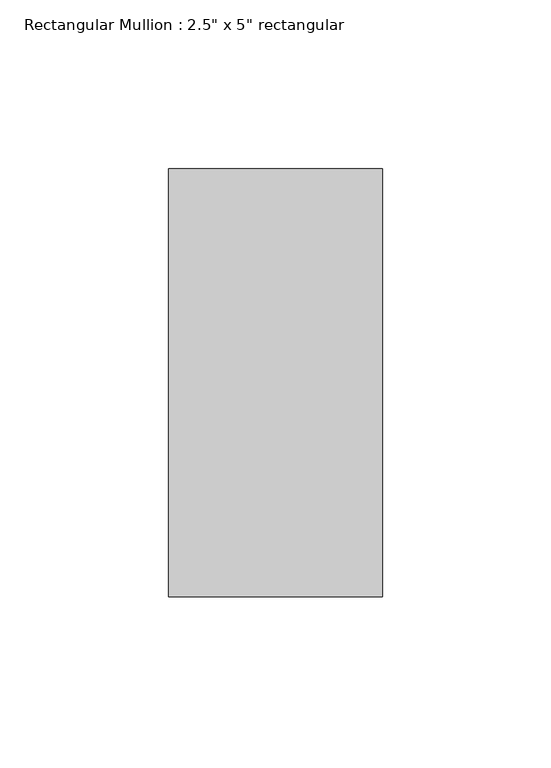
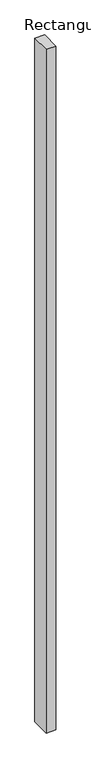
"""IFC4 building model written with IfcOpenShell, lengths in millimetres: member geometry."""

from ifc_helpers import new_model, si_unit, frame, origin, place, context, project, spatial, polyline, outline, extrude, source, transform, mapped, element, save


def member_bf9e663f(model_context):
    return source(origin(), model_context, "Body", "SweptSolid", [
        extrude(outline(polyline([(0.0, 63.5), (0.0, -63.5), (-63.5, -63.5), (-63.5, 63.5), (0.0, 63.5)])), frame((0.0, 0.0, -4736.2841492), z_axis=(0.0, 0.0, 1.0), x_axis=(1.0, 0.0, 0.0)), (0.0, 0.0, 1.0), 4736.2841492),
    ])


if __name__ == "__main__":
    model = new_model("IFC4")
    model_context = context("Model", 3, world=origin())
    ifc_project = project(units=[si_unit("LENGTHUNIT", "METRE", prefix="MILLI")], contexts=[model_context])
    site = spatial("IfcSite", under=ifc_project)
    building = spatial("IfcBuilding", under=site)
    placement = place(None, origin())
    member_shape = member_bf9e663f(model_context)
    element("IfcMember", 1, ObjectType="Rectangular Mullion : 2.5\" x 5\" rectangular", at=placement, inside=building, context=model_context, shape_type="MappedRepresentation", body=[
        mapped(member_shape, transform((0.0, 0.0, 0.0), x_axis=(1.0, 0.0, 0.0), y_axis=(0.0, 1.0, 0.0), z_axis=(0.0, 0.0, 1.0))),
    ])
    save(model, "model.ifc")

# Revit data of these elements
# Type "Rectangular Mullion : 2.5\" x 5\" rectangular"
#   built-in parameter 1007304 = 0.416667 (stored number, unit not read)
#   built-in parameter 1007301 = 0.104167 (stored number, unit not read)
#   built-in parameter 1007300 = 0.104167 (stored number, unit not read)
# Element 1 (IfcMember, "Rectangular Mullion : 2.5\" x 5\" rectangular")
#   Materials on its faces: "Aluminum"
# Materials
#   "Aluminum": class "Metal", colour RGB 247 247 247, transparency 0, Description = "Aluminum 6061", Cost = 0
